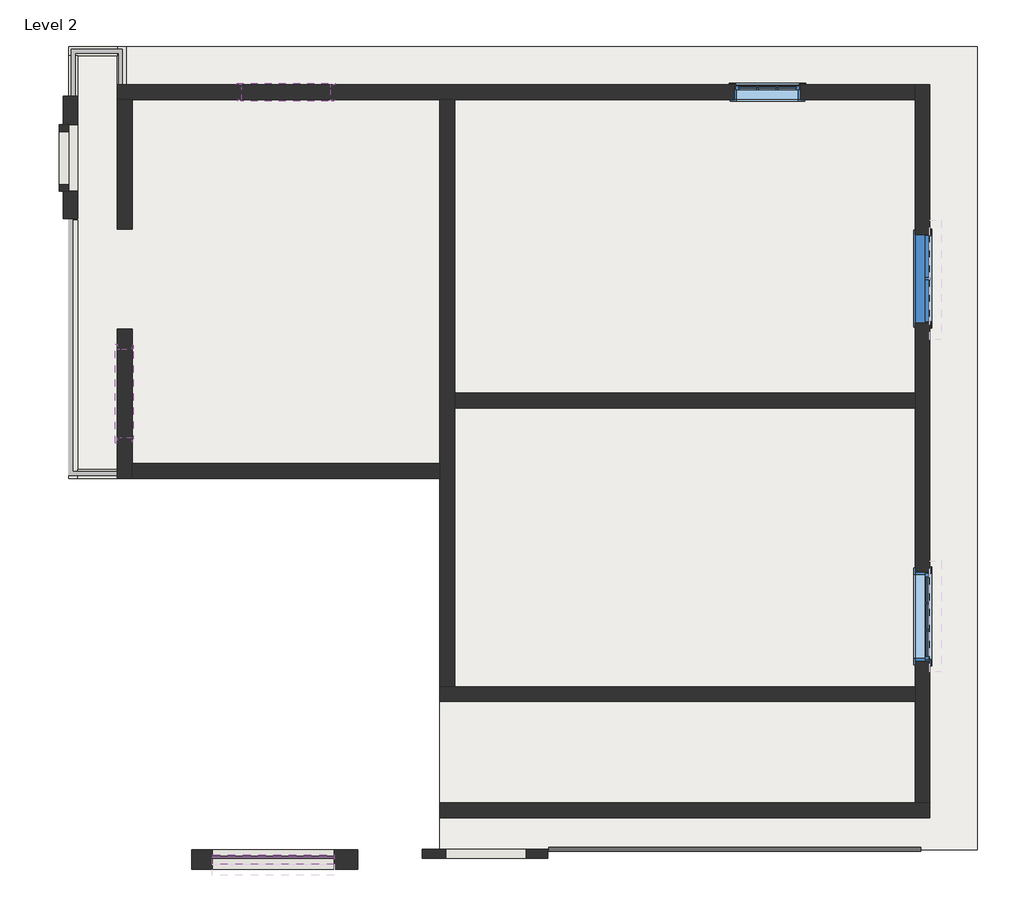
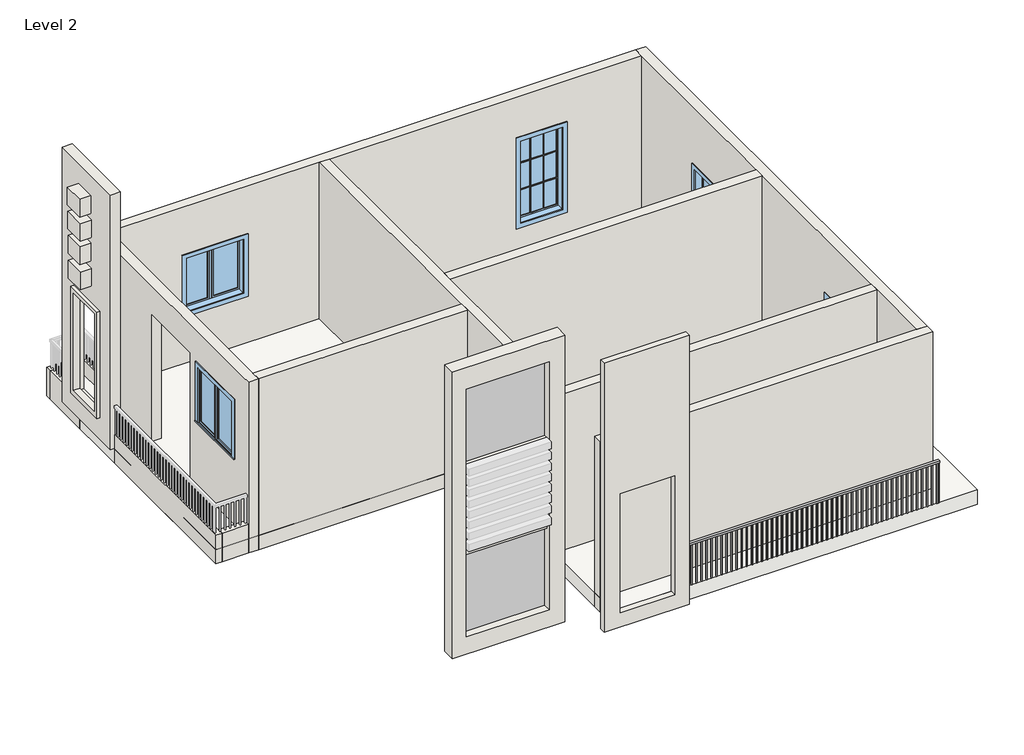
# One storey, part 1 of 2: 17 walls, 5 windows, 2 plates, 1 railing, 1 roof.
"""IFC4 building model written with IfcOpenShell, lengths in millimetres."""

from ifc_helpers import new_model, si_unit, frame, origin, place, context, project, spatial, polyline, outline, extrude, faceted_brep, transform, mapped, element, save
from components import system_panel_glazed_a1eab1ce, system_panel_glazed_1654ed80, walls_3_walls_3_431fb133, walls_4_walls_4_b785277b, window_8b323df3, window_26ecbd3e, window_0862ab64

model = new_model("IFC4")

# Units and contexts
model_context = context("Model", 3, world=origin())
ifc_project = project(units=[si_unit("LENGTHUNIT", "METRE", prefix="MILLI")], contexts=[model_context])

# Site, building, storey
site = spatial("IfcSite", under=ifc_project)
building = spatial("IfcBuilding", under=site)
storey = spatial("IfcBuildingStorey", under=building, Name="Level 2", Elevation=3657.6)

# Plates
placement = place(None, origin())
system_panel_glazed_shape = system_panel_glazed_a1eab1ce(model_context)
element("IfcPlate", 1, ObjectType="System Panel : Glazed", at=placement, inside=storey, context=model_context, shape_type="MappedRepresentation", body=[
    mapped(system_panel_glazed_shape, transform((-9639.2344883, -2764.9451776, 4624.9845939), x_axis=(1.0, 0.0, 0.0), y_axis=(0.0, 1.0, 0.0), z_axis=(0.0, 0.0, 1.0))),
])
system_panel_glazed_2_shape = system_panel_glazed_1654ed80(model_context)
element("IfcPlate", 2, ObjectType="System Panel : Glazed", at=placement, inside=storey, context=model_context, shape_type="MappedRepresentation", body=[
    mapped(system_panel_glazed_2_shape, transform((-9639.2344883, -2764.9451776, 8296.7838361), x_axis=(1.0, 0.0, 0.0), y_axis=(0.0, 1.0, 0.0), z_axis=(0.0, 0.0, 1.0))),
])

# Railing
element("IfcRailing", 3, ObjectType="Handrail - Rectangular", at=placement, inside=storey, context=model_context, shape_type="SweptSolid", body=[
    extrude(outline(polyline([(-5852.0641548, -2650.200333), (-5852.0641548, -2599.400333), (-736.6496253, -2599.400333), (-736.6496253, -2650.200333), (-5852.0641548, -2650.200333)])), frame((0.0, 0.0, 4826.0), z_axis=(0.0, 0.0, 1.0), x_axis=(1.0, 0.0, 0.0)), (0.0, 0.0, 1.0), 50.8),
    extrude(outline(polyline([(-781.5891548, -2634.325333), (-781.5891548, -2615.275333), (-762.5391548, -2615.275333), (-762.5391548, -2634.325333), (-781.5891548, -2634.325333)])), frame((0.0, 0.0, 3962.4), z_axis=(0.0, 0.0, 1.0), x_axis=(1.0, 0.0, 0.0)), (0.0, 0.0, 1.0), 863.6),
    extrude(outline(polyline([(-883.1891548, -2634.325333), (-883.1891548, -2615.275333), (-864.1391548, -2615.275333), (-864.1391548, -2634.325333), (-883.1891548, -2634.325333)])), frame((0.0, 0.0, 3962.4), z_axis=(0.0, 0.0, 1.0), x_axis=(1.0, 0.0, 0.0)), (0.0, 0.0, 1.0), 863.6),
    extrude(outline(polyline([(-984.7891548, -2634.325333), (-984.7891548, -2615.275333), (-965.7391548, -2615.275333), (-965.7391548, -2634.325333), (-984.7891548, -2634.325333)])), frame((0.0, 0.0, 3962.4), z_axis=(0.0, 0.0, 1.0), x_axis=(1.0, 0.0, 0.0)), (0.0, 0.0, 1.0), 863.6),
    extrude(outline(polyline([(-1086.3891548, -2634.325333), (-1086.3891548, -2615.275333), (-1067.3391548, -2615.275333), (-1067.3391548, -2634.325333), (-1086.3891548, -2634.325333)])), frame((0.0, 0.0, 3962.4), z_axis=(0.0, 0.0, 1.0), x_axis=(1.0, 0.0, 0.0)), (0.0, 0.0, 1.0), 863.6),
    extrude(outline(polyline([(-1187.9891548, -2634.325333), (-1187.9891548, -2615.275333), (-1168.9391548, -2615.275333), (-1168.9391548, -2634.325333), (-1187.9891548, -2634.325333)])), frame((0.0, 0.0, 3962.4), z_axis=(0.0, 0.0, 1.0), x_axis=(1.0, 0.0, 0.0)), (0.0, 0.0, 1.0), 863.6),
    extrude(outline(polyline([(-1289.5891548, -2634.325333), (-1289.5891548, -2615.275333), (-1270.5391548, -2615.275333), (-1270.5391548, -2634.325333), (-1289.5891548, -2634.325333)])), frame((0.0, 0.0, 3962.4), z_axis=(0.0, 0.0, 1.0), x_axis=(1.0, 0.0, 0.0)), (0.0, 0.0, 1.0), 863.6),
    extrude(outline(polyline([(-1391.1891548, -2634.325333), (-1391.1891548, -2615.275333), (-1372.1391548, -2615.275333), (-1372.1391548, -2634.325333), (-1391.1891548, -2634.325333)])), frame((0.0, 0.0, 3962.4), z_axis=(0.0, 0.0, 1.0), x_axis=(1.0, 0.0, 0.0)), (0.0, 0.0, 1.0), 863.6),
    extrude(outline(polyline([(-1492.7891548, -2634.325333), (-1492.7891548, -2615.275333), (-1473.7391548, -2615.275333), (-1473.7391548, -2634.325333), (-1492.7891548, -2634.325333)])), frame((0.0, 0.0, 3962.4), z_axis=(0.0, 0.0, 1.0), x_axis=(1.0, 0.0, 0.0)), (0.0, 0.0, 1.0), 863.6),
    extrude(outline(polyline([(-1594.3891548, -2634.325333), (-1594.3891548, -2615.275333), (-1575.3391548, -2615.275333), (-1575.3391548, -2634.325333), (-1594.3891548, -2634.325333)])), frame((0.0, 0.0, 3962.4), z_axis=(0.0, 0.0, 1.0), x_axis=(1.0, 0.0, 0.0)), (0.0, 0.0, 1.0), 863.6),
    extrude(outline(polyline([(-1695.9891548, -2634.325333), (-1695.9891548, -2615.275333), (-1676.9391548, -2615.275333), (-1676.9391548, -2634.325333), (-1695.9891548, -2634.325333)])), frame((0.0, 0.0, 3962.4), z_axis=(0.0, 0.0, 1.0), x_axis=(1.0, 0.0, 0.0)), (0.0, 0.0, 1.0), 863.6),
    extrude(outline(polyline([(-1797.5891548, -2634.325333), (-1797.5891548, -2615.275333), (-1778.5391548, -2615.275333), (-1778.5391548, -2634.325333), (-1797.5891548, -2634.325333)])), frame((0.0, 0.0, 3962.4), z_axis=(0.0, 0.0, 1.0), x_axis=(1.0, 0.0, 0.0)), (0.0, 0.0, 1.0), 863.6),
    extrude(outline(polyline([(-1899.1891548, -2634.325333), (-1899.1891548, -2615.275333), (-1880.1391548, -2615.275333), (-1880.1391548, -2634.325333), (-1899.1891548, -2634.325333)])), frame((0.0, 0.0, 3962.4), z_axis=(0.0, 0.0, 1.0), x_axis=(1.0, 0.0, 0.0)), (0.0, 0.0, 1.0), 863.6),
    extrude(outline(polyline([(-2000.7891548, -2634.325333), (-2000.7891548, -2615.275333), (-1981.7391548, -2615.275333), (-1981.7391548, -2634.325333), (-2000.7891548, -2634.325333)])), frame((0.0, 0.0, 3962.4), z_axis=(0.0, 0.0, 1.0), x_axis=(1.0, 0.0, 0.0)), (0.0, 0.0, 1.0), 863.6),
    extrude(outline(polyline([(-2102.3891548, -2634.325333), (-2102.3891548, -2615.275333), (-2083.3391548, -2615.275333), (-2083.3391548, -2634.325333), (-2102.3891548, -2634.325333)])), frame((0.0, 0.0, 3962.4), z_axis=(0.0, 0.0, 1.0), x_axis=(1.0, 0.0, 0.0)), (0.0, 0.0, 1.0), 863.6),
    extrude(outline(polyline([(-2203.9891548, -2634.325333), (-2203.9891548, -2615.275333), (-2184.9391548, -2615.275333), (-2184.9391548, -2634.325333), (-2203.9891548, -2634.325333)])), frame((0.0, 0.0, 3962.4), z_axis=(0.0, 0.0, 1.0), x_axis=(1.0, 0.0, 0.0)), (0.0, 0.0, 1.0), 863.6),
    extrude(outline(polyline([(-2305.5891548, -2634.325333), (-2305.5891548, -2615.275333), (-2286.5391548, -2615.275333), (-2286.5391548, -2634.325333), (-2305.5891548, -2634.325333)])), frame((0.0, 0.0, 3962.4), z_axis=(0.0, 0.0, 1.0), x_axis=(1.0, 0.0, 0.0)), (0.0, 0.0, 1.0), 863.6),
    extrude(outline(polyline([(-2407.1891548, -2634.325333), (-2407.1891548, -2615.275333), (-2388.1391548, -2615.275333), (-2388.1391548, -2634.325333), (-2407.1891548, -2634.325333)])), frame((0.0, 0.0, 3962.4), z_axis=(0.0, 0.0, 1.0), x_axis=(1.0, 0.0, 0.0)), (0.0, 0.0, 1.0), 863.6),
    extrude(outline(polyline([(-2508.7891548, -2634.325333), (-2508.7891548, -2615.275333), (-2489.7391548, -2615.275333), (-2489.7391548, -2634.325333), (-2508.7891548, -2634.325333)])), frame((0.0, 0.0, 3962.4), z_axis=(0.0, 0.0, 1.0), x_axis=(1.0, 0.0, 0.0)), (0.0, 0.0, 1.0), 863.6),
    extrude(outline(polyline([(-2610.3891548, -2634.325333), (-2610.3891548, -2615.275333), (-2591.3391548, -2615.275333), (-2591.3391548, -2634.325333), (-2610.3891548, -2634.325333)])), frame((0.0, 0.0, 3962.4), z_axis=(0.0, 0.0, 1.0), x_axis=(1.0, 0.0, 0.0)), (0.0, 0.0, 1.0), 863.6),
    extrude(outline(polyline([(-2711.9891548, -2634.325333), (-2711.9891548, -2615.275333), (-2692.9391548, -2615.275333), (-2692.9391548, -2634.325333), (-2711.9891548, -2634.325333)])), frame((0.0, 0.0, 3962.4), z_axis=(0.0, 0.0, 1.0), x_axis=(1.0, 0.0, 0.0)), (0.0, 0.0, 1.0), 863.6),
    extrude(outline(polyline([(-2813.5891548, -2634.325333), (-2813.5891548, -2615.275333), (-2794.5391548, -2615.275333), (-2794.5391548, -2634.325333), (-2813.5891548, -2634.325333)])), frame((0.0, 0.0, 3962.4), z_axis=(0.0, 0.0, 1.0), x_axis=(1.0, 0.0, 0.0)), (0.0, 0.0, 1.0), 863.6),
    extrude(outline(polyline([(-2915.1891548, -2634.325333), (-2915.1891548, -2615.275333), (-2896.1391548, -2615.275333), (-2896.1391548, -2634.325333), (-2915.1891548, -2634.325333)])), frame((0.0, 0.0, 3962.4), z_axis=(0.0, 0.0, 1.0), x_axis=(1.0, 0.0, 0.0)), (0.0, 0.0, 1.0), 863.6),
    extrude(outline(polyline([(-3016.7891548, -2634.325333), (-3016.7891548, -2615.275333), (-2997.7391548, -2615.275333), (-2997.7391548, -2634.325333), (-3016.7891548, -2634.325333)])), frame((0.0, 0.0, 3962.4), z_axis=(0.0, 0.0, 1.0), x_axis=(1.0, 0.0, 0.0)), (0.0, 0.0, 1.0), 863.6),
    extrude(outline(polyline([(-3118.3891548, -2634.325333), (-3118.3891548, -2615.275333), (-3099.3391548, -2615.275333), (-3099.3391548, -2634.325333), (-3118.3891548, -2634.325333)])), frame((0.0, 0.0, 3962.4), z_axis=(0.0, 0.0, 1.0), x_axis=(1.0, 0.0, 0.0)), (0.0, 0.0, 1.0), 863.6),
    extrude(outline(polyline([(-3219.9891548, -2634.325333), (-3219.9891548, -2615.275333), (-3200.9391548, -2615.275333), (-3200.9391548, -2634.325333), (-3219.9891548, -2634.325333)])), frame((0.0, 0.0, 3962.4), z_axis=(0.0, 0.0, 1.0), x_axis=(1.0, 0.0, 0.0)), (0.0, 0.0, 1.0), 863.6),
    extrude(outline(polyline([(-3321.5891548, -2634.325333), (-3321.5891548, -2615.275333), (-3302.5391548, -2615.275333), (-3302.5391548, -2634.325333), (-3321.5891548, -2634.325333)])), frame((0.0, 0.0, 3962.4), z_axis=(0.0, 0.0, 1.0), x_axis=(1.0, 0.0, 0.0)), (0.0, 0.0, 1.0), 863.6),
    extrude(outline(polyline([(-3423.1891548, -2634.325333), (-3423.1891548, -2615.275333), (-3404.1391548, -2615.275333), (-3404.1391548, -2634.325333), (-3423.1891548, -2634.325333)])), frame((0.0, 0.0, 3962.4), z_axis=(0.0, 0.0, 1.0), x_axis=(1.0, 0.0, 0.0)), (0.0, 0.0, 1.0), 863.6),
    extrude(outline(polyline([(-3524.7891548, -2634.325333), (-3524.7891548, -2615.275333), (-3505.7391548, -2615.275333), (-3505.7391548, -2634.325333), (-3524.7891548, -2634.325333)])), frame((0.0, 0.0, 3962.4), z_axis=(0.0, 0.0, 1.0), x_axis=(1.0, 0.0, 0.0)), (0.0, 0.0, 1.0), 863.6),
    extrude(outline(polyline([(-3626.3891548, -2634.325333), (-3626.3891548, -2615.275333), (-3607.3391548, -2615.275333), (-3607.3391548, -2634.325333), (-3626.3891548, -2634.325333)])), frame((0.0, 0.0, 3962.4), z_axis=(0.0, 0.0, 1.0), x_axis=(1.0, 0.0, 0.0)), (0.0, 0.0, 1.0), 863.6),
    extrude(outline(polyline([(-3727.9891548, -2634.325333), (-3727.9891548, -2615.275333), (-3708.9391548, -2615.275333), (-3708.9391548, -2634.325333), (-3727.9891548, -2634.325333)])), frame((0.0, 0.0, 3962.4), z_axis=(0.0, 0.0, 1.0), x_axis=(1.0, 0.0, 0.0)), (0.0, 0.0, 1.0), 863.6),
    extrude(outline(polyline([(-3829.5891548, -2634.325333), (-3829.5891548, -2615.275333), (-3810.5391548, -2615.275333), (-3810.5391548, -2634.325333), (-3829.5891548, -2634.325333)])), frame((0.0, 0.0, 3962.4), z_axis=(0.0, 0.0, 1.0), x_axis=(1.0, 0.0, 0.0)), (0.0, 0.0, 1.0), 863.6),
    extrude(outline(polyline([(-3931.1891548, -2634.325333), (-3931.1891548, -2615.275333), (-3912.1391548, -2615.275333), (-3912.1391548, -2634.325333), (-3931.1891548, -2634.325333)])), frame((0.0, 0.0, 3962.4), z_axis=(0.0, 0.0, 1.0), x_axis=(1.0, 0.0, 0.0)), (0.0, 0.0, 1.0), 863.6),
    extrude(outline(polyline([(-4032.7891548, -2634.325333), (-4032.7891548, -2615.275333), (-4013.7391548, -2615.275333), (-4013.7391548, -2634.325333), (-4032.7891548, -2634.325333)])), frame((0.0, 0.0, 3962.4), z_axis=(0.0, 0.0, 1.0), x_axis=(1.0, 0.0, 0.0)), (0.0, 0.0, 1.0), 863.6),
    extrude(outline(polyline([(-4134.3891548, -2634.325333), (-4134.3891548, -2615.275333), (-4115.3391548, -2615.275333), (-4115.3391548, -2634.325333), (-4134.3891548, -2634.325333)])), frame((0.0, 0.0, 3962.4), z_axis=(0.0, 0.0, 1.0), x_axis=(1.0, 0.0, 0.0)), (0.0, 0.0, 1.0), 863.6),
    extrude(outline(polyline([(-4235.9891548, -2634.325333), (-4235.9891548, -2615.275333), (-4216.9391548, -2615.275333), (-4216.9391548, -2634.325333), (-4235.9891548, -2634.325333)])), frame((0.0, 0.0, 3962.4), z_axis=(0.0, 0.0, 1.0), x_axis=(1.0, 0.0, 0.0)), (0.0, 0.0, 1.0), 863.6),
    extrude(outline(polyline([(-4337.5891548, -2634.325333), (-4337.5891548, -2615.275333), (-4318.5391548, -2615.275333), (-4318.5391548, -2634.325333), (-4337.5891548, -2634.325333)])), frame((0.0, 0.0, 3962.4), z_axis=(0.0, 0.0, 1.0), x_axis=(1.0, 0.0, 0.0)), (0.0, 0.0, 1.0), 863.6),
    extrude(outline(polyline([(-4439.1891548, -2634.325333), (-4439.1891548, -2615.275333), (-4420.1391548, -2615.275333), (-4420.1391548, -2634.325333), (-4439.1891548, -2634.325333)])), frame((0.0, 0.0, 3962.4), z_axis=(0.0, 0.0, 1.0), x_axis=(1.0, 0.0, 0.0)), (0.0, 0.0, 1.0), 863.6),
    extrude(outline(polyline([(-4540.7891548, -2634.325333), (-4540.7891548, -2615.275333), (-4521.7391548, -2615.275333), (-4521.7391548, -2634.325333), (-4540.7891548, -2634.325333)])), frame((0.0, 0.0, 3962.4), z_axis=(0.0, 0.0, 1.0), x_axis=(1.0, 0.0, 0.0)), (0.0, 0.0, 1.0), 863.6),
    extrude(outline(polyline([(-4642.3891548, -2634.325333), (-4642.3891548, -2615.275333), (-4623.3391548, -2615.275333), (-4623.3391548, -2634.325333), (-4642.3891548, -2634.325333)])), frame((0.0, 0.0, 3962.4), z_axis=(0.0, 0.0, 1.0), x_axis=(1.0, 0.0, 0.0)), (0.0, 0.0, 1.0), 863.6),
    extrude(outline(polyline([(-4743.9891548, -2634.325333), (-4743.9891548, -2615.275333), (-4724.9391548, -2615.275333), (-4724.9391548, -2634.325333), (-4743.9891548, -2634.325333)])), frame((0.0, 0.0, 3962.4), z_axis=(0.0, 0.0, 1.0), x_axis=(1.0, 0.0, 0.0)), (0.0, 0.0, 1.0), 863.6),
    extrude(outline(polyline([(-4845.5891548, -2634.325333), (-4845.5891548, -2615.275333), (-4826.5391548, -2615.275333), (-4826.5391548, -2634.325333), (-4845.5891548, -2634.325333)])), frame((0.0, 0.0, 3962.4), z_axis=(0.0, 0.0, 1.0), x_axis=(1.0, 0.0, 0.0)), (0.0, 0.0, 1.0), 863.6),
    extrude(outline(polyline([(-4947.1891548, -2634.325333), (-4947.1891548, -2615.275333), (-4928.1391548, -2615.275333), (-4928.1391548, -2634.325333), (-4947.1891548, -2634.325333)])), frame((0.0, 0.0, 3962.4), z_axis=(0.0, 0.0, 1.0), x_axis=(1.0, 0.0, 0.0)), (0.0, 0.0, 1.0), 863.6),
    extrude(outline(polyline([(-5048.7891548, -2634.325333), (-5048.7891548, -2615.275333), (-5029.7391548, -2615.275333), (-5029.7391548, -2634.325333), (-5048.7891548, -2634.325333)])), frame((0.0, 0.0, 3962.4), z_axis=(0.0, 0.0, 1.0), x_axis=(1.0, 0.0, 0.0)), (0.0, 0.0, 1.0), 863.6),
    extrude(outline(polyline([(-5150.3891548, -2634.325333), (-5150.3891548, -2615.275333), (-5131.3391548, -2615.275333), (-5131.3391548, -2634.325333), (-5150.3891548, -2634.325333)])), frame((0.0, 0.0, 3962.4), z_axis=(0.0, 0.0, 1.0), x_axis=(1.0, 0.0, 0.0)), (0.0, 0.0, 1.0), 863.6),
    extrude(outline(polyline([(-5251.9891548, -2634.325333), (-5251.9891548, -2615.275333), (-5232.9391548, -2615.275333), (-5232.9391548, -2634.325333), (-5251.9891548, -2634.325333)])), frame((0.0, 0.0, 3962.4), z_axis=(0.0, 0.0, 1.0), x_axis=(1.0, 0.0, 0.0)), (0.0, 0.0, 1.0), 863.6),
    extrude(outline(polyline([(-5353.5891548, -2634.325333), (-5353.5891548, -2615.275333), (-5334.5391548, -2615.275333), (-5334.5391548, -2634.325333), (-5353.5891548, -2634.325333)])), frame((0.0, 0.0, 3962.4), z_axis=(0.0, 0.0, 1.0), x_axis=(1.0, 0.0, 0.0)), (0.0, 0.0, 1.0), 863.6),
    extrude(outline(polyline([(-5455.1891548, -2634.325333), (-5455.1891548, -2615.275333), (-5436.1391548, -2615.275333), (-5436.1391548, -2634.325333), (-5455.1891548, -2634.325333)])), frame((0.0, 0.0, 3962.4), z_axis=(0.0, 0.0, 1.0), x_axis=(1.0, 0.0, 0.0)), (0.0, 0.0, 1.0), 863.6),
    extrude(outline(polyline([(-5556.7891548, -2634.325333), (-5556.7891548, -2615.275333), (-5537.7391548, -2615.275333), (-5537.7391548, -2634.325333), (-5556.7891548, -2634.325333)])), frame((0.0, 0.0, 3962.4), z_axis=(0.0, 0.0, 1.0), x_axis=(1.0, 0.0, 0.0)), (0.0, 0.0, 1.0), 863.6),
    extrude(outline(polyline([(-5658.3891548, -2634.325333), (-5658.3891548, -2615.275333), (-5639.3391548, -2615.275333), (-5639.3391548, -2634.325333), (-5658.3891548, -2634.325333)])), frame((0.0, 0.0, 3962.4), z_axis=(0.0, 0.0, 1.0), x_axis=(1.0, 0.0, 0.0)), (0.0, 0.0, 1.0), 863.6),
    extrude(outline(polyline([(-5759.9891548, -2634.325333), (-5759.9891548, -2615.275333), (-5740.9391548, -2615.275333), (-5740.9391548, -2634.325333), (-5759.9891548, -2634.325333)])), frame((0.0, 0.0, 3962.4), z_axis=(0.0, 0.0, 1.0), x_axis=(1.0, 0.0, 0.0)), (0.0, 0.0, 1.0), 863.6),
    extrude(outline(polyline([(-755.6996253, -2634.325333), (-755.6996253, -2615.275333), (-736.6496253, -2615.275333), (-736.6496253, -2634.325333), (-755.6996253, -2634.325333)])), frame((0.0, 0.0, 3962.4), z_axis=(0.0, 0.0, 1.0), x_axis=(1.0, 0.0, 0.0)), (0.0, 0.0, 1.0), 863.6),
    extrude(outline(polyline([(-5852.0641548, -2634.325333), (-5852.0641548, -2615.275333), (-5833.0141548, -2615.275333), (-5833.0141548, -2634.325333), (-5852.0641548, -2634.325333)])), frame((0.0, 0.0, 3962.4), z_axis=(0.0, 0.0, 1.0), x_axis=(1.0, 0.0, 0.0)), (0.0, 0.0, 1.0), 863.6),
])

# Roof
element("IfcRoof", 4, ObjectType="Generic - 12\"", at=placement, inside=storey, context=model_context, shape_type="SweptSolid", body=[
    extrude(outline(polyline([(-12453.9083357, 8420.5483652), (42.8916643, 8420.5483652), (42.8916643, -2628.4516348), (-7348.5083357, -2628.4516348), (-7348.5083357, 2476.9483652), (-12453.9083357, 2476.9483652), (-12453.9083357, 8420.5483652)])), frame((0.0, 0.0, 3657.6), z_axis=(0.0, 0.0, 1.0), x_axis=(1.0, 0.0, 0.0)), (0.0, 0.0, 1.0), 304.8),
])

# Walls
element("IfcWall", 5, ObjectType="Generic - 5\"", at=placement, inside=storey, context=model_context, shape_type="SweptSolid", body=[
    extrude(outline(polyline([(3657.6, -7595.2932708), (3657.6, -5868.0932708), (9420.9325813, -5868.0932708), (9420.9325813, -7595.2932708), (3657.6, -7595.2932708)]), holes=[polyline([(6512.6251814, -6163.3682708), (3962.4, -6163.3682708), (3962.4, -7272.3083357), (6512.6251814, -7272.3083357), (6512.6251814, -6163.3682708)])]), frame((0.0, -2750.326099, 0.0), z_axis=(0.0, 1.0, 0.0), x_axis=(0.0, 0.0, 1.0)), (0.0, 0.0, 1.0), 127.0),
])
element("IfcWall", 6, ObjectType="Generic - 5\"", at=placement, inside=storey, context=model_context, shape_type="Brep", body=[
    faceted_brep([(-11659.2932708, 7892.273901, 3657.6), (-11659.2932708, 8420.5483652, 3657.6), (-11659.2932708, 8420.5483652, 4267.2), (-11659.2932708, 7892.273901, 4267.2), (-11786.2932708, 7892.273901, 3657.6), (-11786.2932708, 7892.273901, 4267.2), (-11786.2932708, 8293.5483652, 4267.2), (-11786.2932708, 8420.5483652, 4267.2), (-11786.2932708, 8420.5483652, 3657.6), (-11786.2932708, 8293.5483652, 3657.6)], [[[0, 1, 2, 3]], [[4, 5, 6, 7, 8, 9]], [[1, 0, 4, 9, 8]], [[3, 2, 7, 6, 5]], [[0, 3, 5, 4]], [[2, 1, 8, 7]]]),
])
element("IfcWall", 7, ObjectType="Generic - 5\"", at=placement, inside=storey, context=model_context, shape_type="Brep", body=[
    faceted_brep([(-11786.2932708, 8420.5483652, 3657.6), (-12453.9083357, 8420.5483652, 3657.6), (-12453.9083357, 8420.5483652, 4267.2), (-11786.2932708, 8420.5483652, 4267.2), (-11786.2932708, 8293.5483652, 3657.6), (-11786.2932708, 8293.5483652, 4267.2), (-12326.9083357, 8293.5483652, 4267.2), (-12453.9083357, 8293.5483652, 4267.2), (-12453.9083357, 8293.5483652, 3657.6), (-12326.9083357, 8293.5483652, 3657.6)], [[[0, 1, 2, 3]], [[4, 5, 6, 7, 8, 9]], [[1, 0, 4, 9, 8]], [[3, 2, 7, 6, 5]], [[0, 3, 5, 4]], [[2, 1, 8, 7]]]),
])
element("IfcWall", 8, ObjectType="Generic - 5\"", at=placement, inside=storey, context=model_context, shape_type="SweptSolid", body=[
    extrude(outline(polyline([(-12453.9083357, 7251.0434239), (-12453.9083357, 8293.5483652), (-12326.9083357, 8293.5483652), (-12326.9083357, 7251.0434239), (-12453.9083357, 7251.0434239)])), frame((0.0, 0.0, 3657.6), z_axis=(0.0, 0.0, 1.0), x_axis=(1.0, 0.0, 0.0)), (0.0, 0.0, 1.0), 609.6),
])
element("IfcWall", 9, ObjectType="Generic - 5\"", at=placement, inside=storey, context=model_context, shape_type="Brep", body=[
    faceted_brep([(-12453.9083357, 6032.9483652, 3657.6), (-12453.9083357, 2476.9483652, 3657.6), (-12453.9083357, 2476.9483652, 4267.2), (-12453.9083357, 6032.9483652, 4267.2), (-12326.9083357, 6032.9483652, 3657.6), (-12326.9083357, 6032.9483652, 4267.2), (-12326.9083357, 2603.9483652, 4267.2), (-12326.9083357, 2476.9483652, 4267.2), (-12326.9083357, 2476.9483652, 3657.6), (-12326.9083357, 2603.9483652, 3657.6)], [[[0, 1, 2, 3]], [[4, 5, 6, 7, 8, 9]], [[1, 0, 4, 9, 8]], [[3, 2, 7, 6, 5]], [[0, 3, 5, 4]], [[2, 1, 8, 7]]]),
])
element("IfcWall", 10, ObjectType="Generic - 5\"", at=placement, inside=storey, context=model_context, shape_type="SweptSolid", body=[
    extrude(outline(polyline([(-11786.2932708, 2476.9483652), (-12326.9083357, 2476.9483652), (-12326.9083357, 2603.9483652), (-11786.2932708, 2603.9483652), (-11786.2932708, 2476.9483652)])), frame((0.0, 0.0, 3657.6), z_axis=(0.0, 0.0, 1.0), x_axis=(1.0, 0.0, 0.0)), (0.0, 0.0, 1.0), 609.6),
])
element("IfcWall", 11, ObjectType="Generic - 5\"", at=placement, inside=storey, context=model_context, shape_type="SweptSolid", body=[
    extrude(outline(polyline([(-8801.0344883, -2828.4451776), (-10477.4344883, -2828.4451776), (-10477.4344883, -2701.4451776), (-8801.0344883, -2701.4451776), (-8801.0344883, -2828.4451776)])), frame((0.0, 0.0, 6360.2251814), z_axis=(0.0, 0.0, 1.0), x_axis=(1.0, 0.0, 0.0)), (0.0, 0.0, 1.0), 1936.5586547),
])
element("IfcWall", 12, ObjectType="Generic - 8\"", at=placement, inside=storey, context=model_context, shape_type="Brep", body=[
    faceted_brep([(-11786.2932708, 7689.073901, 7315.2), (-11786.2932708, 7689.073901, 3657.6), (-11583.0932708, 7689.073901, 3657.6), (-7348.5083357, 7689.073901, 3657.6), (-7145.3083357, 7689.073901, 3657.6), (-813.4932708, 7689.073901, 3657.6), (-813.4932708, 7689.073901, 7315.2), (-7145.3083357, 7689.073901, 7315.2), (-7348.5083357, 7689.073901, 7315.2), (-11583.0932708, 7689.073901, 7315.2), (-2388.2932708, 7689.073901, 6386.5202928), (-2388.2932708, 7689.073901, 4557.7202928), (-3302.6932708, 7689.073901, 4557.7202928), (-3302.6932708, 7689.073901, 6386.5202928), (-8856.2008033, 7689.073901, 6244.272578), (-8856.2008033, 7689.073901, 5025.072578), (-10075.4008033, 7689.073901, 5025.072578), (-10075.4008033, 7689.073901, 6244.272578), (-11786.2932708, 7892.273901, 3657.6), (-11786.2932708, 7892.273901, 4267.2), (-11786.2932708, 7892.273901, 7315.2), (-813.4932708, 7892.273901, 7315.2), (-813.4932708, 7892.273901, 3657.6), (-11659.2932708, 7892.273901, 3657.6), (-2388.2932708, 7892.273901, 6386.5202928), (-3302.6932708, 7892.273901, 6386.5202928), (-3302.6932708, 7892.273901, 4557.7202928), (-2388.2932708, 7892.273901, 4557.7202928), (-8856.2008033, 7892.273901, 6244.272578), (-10075.4008033, 7892.273901, 6244.272578), (-10075.4008033, 7892.273901, 5025.072578), (-8856.2008033, 7892.273901, 5025.072578)], [[[0, 1, 2, 3, 4, 5, 6, 7, 8, 9], [10, 11, 12, 13], [14, 15, 16, 17]], [[18, 19, 20, 21, 22, 23], [24, 25, 26, 27], [28, 29, 30, 31]], [[5, 4, 3, 2, 1, 18, 23, 22]], [[0, 9, 8, 7, 6, 21, 20]], [[6, 5, 22, 21]], [[0, 20, 19, 18, 1]], [[11, 10, 24, 27]], [[12, 11, 27, 26]], [[13, 12, 26, 25]], [[10, 13, 25, 24]], [[15, 14, 28, 31]], [[16, 15, 31, 30]], [[17, 16, 30, 29]], [[14, 17, 29, 28]]]),
])
element("IfcWall", 13, ObjectType="Generic - 8\"", at=placement, inside=storey, context=model_context, shape_type="Brep", body=[
    faceted_brep([(-11583.0932708, 2476.9483652, 7315.2), (-11583.0932708, 2476.9483652, 3657.6), (-11583.0932708, 2578.5483652, 3657.6), (-11583.0932708, 2680.1483652, 3657.6), (-11583.0932708, 4533.8772304, 3657.6), (-11583.0932708, 4533.8772304, 6705.6), (-11583.0932708, 5905.4772304, 6705.6), (-11583.0932708, 5905.4772304, 3657.6), (-11583.0932708, 7689.073901, 3657.6), (-11583.0932708, 7689.073901, 7315.2), (-11583.0932708, 2680.1483652, 7315.2), (-11583.0932708, 4254.9483652, 6584.0797977), (-11583.0932708, 4254.9483652, 5364.8797977), (-11583.0932708, 3035.7483652, 5364.8797977), (-11583.0932708, 3035.7483652, 6584.0797977), (-11786.2932708, 2476.9483652, 3657.6), (-11786.2932708, 2476.9483652, 4267.2), (-11786.2932708, 2476.9483652, 7315.2), (-11786.2932708, 2680.1483652, 7315.2), (-11786.2932708, 7689.073901, 7315.2), (-11786.2932708, 7689.073901, 3657.6), (-11786.2932708, 5905.4772304, 3657.6), (-11786.2932708, 5905.4772304, 6705.6), (-11786.2932708, 4533.8772304, 6705.6), (-11786.2932708, 4533.8772304, 3657.6), (-11786.2932708, 2603.9483652, 3657.6), (-11786.2932708, 2578.5483652, 3657.6), (-11786.2932708, 4254.9483652, 6584.0797977), (-11786.2932708, 3035.7483652, 6584.0797977), (-11786.2932708, 3035.7483652, 5364.8797977), (-11786.2932708, 4254.9483652, 5364.8797977)], [[[0, 1, 2, 3, 4, 5, 6, 7, 8, 9, 10], [11, 12, 13, 14]], [[15, 16, 17, 18, 19, 20, 21, 22, 23, 24, 25, 26], [27, 28, 29, 30]], [[0, 17, 16, 15, 1]], [[8, 20, 19, 9]], [[12, 11, 27, 30]], [[13, 12, 30, 29]], [[14, 13, 29, 28]], [[11, 14, 28, 27]], [[0, 10, 9, 19, 18, 17]], [[4, 3, 2, 1, 15, 26, 25, 24]], [[5, 4, 24, 23]], [[6, 5, 23, 22]], [[7, 6, 22, 21]], [[8, 7, 21, 20]]]),
])
element("IfcWall", 14, ObjectType="Generic - 8\"", at=placement, inside=storey, context=model_context, shape_type="Brep", body=[
    faceted_brep([(-610.2932708, -1988.326099, 3657.6), (-813.4932708, -1988.326099, 3657.6), (-7348.5083357, -1988.326099, 3657.6), (-7348.5083357, -1988.326099, 7315.2), (-813.4932708, -1988.326099, 7315.2), (-610.2932708, -1988.326099, 7315.2), (-610.2932708, -2191.526099, 3657.6), (-610.2932708, -2191.526099, 7315.2), (-7348.5083357, -2191.526099, 7315.2), (-7348.5083357, -2191.526099, 3657.6)], [[[0, 1, 2, 3, 4, 5]], [[6, 7, 8, 9]], [[2, 1, 0, 6, 9]], [[3, 2, 9, 8]], [[5, 4, 3, 8, 7]], [[0, 5, 7, 6]]]),
])
element("IfcWall", 15, ObjectType="Generic - 8\"", at=placement, inside=storey, context=model_context, shape_type="Brep", body=[
    faceted_brep([(-813.4932708, 7892.273901, 3657.6), (-813.4932708, 7689.073901, 3657.6), (-813.4932708, 3650.473901, 3657.6), (-813.4932708, 3447.273901, 3657.6), (-813.4932708, -388.126099, 3657.6), (-813.4932708, -591.326099, 3657.6), (-813.4932708, -1988.326099, 3657.6), (-813.4932708, -1988.326099, 7315.2), (-813.4932708, -591.326099, 7315.2), (-813.4932708, -388.126099, 7315.2), (-813.4932708, 3447.273901, 7315.2), (-813.4932708, 3650.473901, 7315.2), (-813.4932708, 7689.073901, 7315.2), (-813.4932708, 7892.273901, 7315.2), (-813.4932708, -32.526099, 6096.0), (-813.4932708, -32.526099, 4572.0), (-813.4932708, 1186.673901, 4572.0), (-813.4932708, 1186.673901, 6096.0), (-813.4932708, 4615.673901, 6045.2), (-813.4932708, 4615.673901, 4826.0), (-813.4932708, 5834.873901, 4826.0), (-813.4932708, 5834.873901, 6045.2), (-610.2932708, 7892.273901, 3657.6), (-610.2932708, 7892.273901, 7315.2), (-610.2932708, -1988.326099, 7315.2), (-610.2932708, -1988.326099, 3657.6), (-610.2932708, -32.526099, 6096.0), (-610.2932708, 1186.673901, 6096.0), (-610.2932708, 1186.673901, 4572.0), (-610.2932708, -32.526099, 4572.0), (-610.2932708, 4615.673901, 6045.2), (-610.2932708, 5834.873901, 6045.2), (-610.2932708, 5834.873901, 4826.0), (-610.2932708, 4615.673901, 4826.0)], [[[0, 1, 2, 3, 4, 5, 6, 7, 8, 9, 10, 11, 12, 13], [14, 15, 16, 17], [18, 19, 20, 21]], [[22, 23, 24, 25], [26, 27, 28, 29], [30, 31, 32, 33]], [[6, 5, 4, 3, 2, 1, 0, 22, 25]], [[13, 12, 11, 10, 9, 8, 7, 24, 23]], [[0, 13, 23, 22]], [[7, 6, 25, 24]], [[15, 14, 26, 29]], [[16, 15, 29, 28]], [[17, 16, 28, 27]], [[14, 17, 27, 26]], [[19, 18, 30, 33]], [[20, 19, 33, 32]], [[21, 20, 32, 31]], [[18, 21, 31, 30]]]),
])
element("IfcWall", 16, ObjectType="Generic - 8\"", at=placement, inside=storey, context=model_context, shape_type="Brep", body=[
    faceted_brep([(-813.4932708, -388.126099, 3657.6), (-7145.3083357, -388.126099, 3657.6), (-7348.5083357, -388.126099, 3657.6), (-7348.5083357, -388.126099, 7315.2), (-7145.3083357, -388.126099, 7315.2), (-813.4932708, -388.126099, 7315.2), (-813.4932708, -591.326099, 3657.6), (-813.4932708, -591.326099, 7315.2), (-7348.5083357, -591.326099, 7315.2), (-7348.5083357, -591.326099, 3657.6)], [[[0, 1, 2, 3, 4, 5]], [[6, 7, 8, 9]], [[2, 1, 0, 6, 9]], [[5, 4, 3, 8, 7]], [[0, 5, 7, 6]], [[3, 2, 9, 8]]]),
])
element("IfcWall", 17, ObjectType="Generic - 8\"", at=placement, inside=storey, context=model_context, shape_type="Brep", body=[
    faceted_brep([(-7145.3083357, -388.126099, 3657.6), (-7145.3083357, 3447.273901, 3657.6), (-7145.3083357, 3650.473901, 3657.6), (-7145.3083357, 7689.073901, 3657.6), (-7145.3083357, 7689.073901, 7315.2), (-7145.3083357, 3650.473901, 7315.2), (-7145.3083357, 3447.273901, 7315.2), (-7145.3083357, -388.126099, 7315.2), (-7348.5083357, -388.126099, 3657.6), (-7348.5083357, -388.126099, 7315.2), (-7348.5083357, 2476.9483652, 7315.2), (-7348.5083357, 2680.1483652, 7315.2), (-7348.5083357, 7689.073901, 7315.2), (-7348.5083357, 7689.073901, 3657.6), (-7348.5083357, 2680.1483652, 3657.6), (-7348.5083357, 2476.9483652, 3657.6)], [[[0, 1, 2, 3, 4, 5, 6, 7]], [[8, 9, 10, 11, 12, 13, 14, 15]], [[3, 2, 1, 0, 8, 15, 14, 13]], [[7, 6, 5, 4, 12, 11, 10, 9]], [[0, 7, 9, 8]], [[4, 3, 13, 12]]]),
])
element("IfcWall", 18, ObjectType="Generic - 8\"", at=placement, inside=storey, context=model_context, shape_type="Brep", body=[
    faceted_brep([(-7348.5083357, 2680.1483652, 3657.6), (-11583.0932708, 2680.1483652, 3657.6), (-11583.0932708, 2680.1483652, 7315.2), (-7366.6932708, 2680.1483652, 7315.2), (-7348.5083357, 2680.1483652, 7315.2), (-7348.5083357, 2476.9483652, 3657.6), (-7348.5083357, 2476.9483652, 7315.2), (-7366.6932708, 2476.9483652, 7315.2), (-11583.0932708, 2476.9483652, 7315.2), (-11583.0932708, 2476.9483652, 3657.6)], [[[0, 1, 2, 3, 4]], [[5, 6, 7, 8, 9]], [[1, 0, 5, 9]], [[4, 3, 2, 8, 7, 6]], [[0, 4, 6, 5]], [[1, 9, 8, 2]]]),
])
element("IfcWall", 19, ObjectType="Generic - 8\"", at=placement, inside=storey, context=model_context, shape_type="SweptSolid", body=[
    extrude(outline(polyline([(-813.4932708, 3447.273901), (-7145.3083357, 3447.273901), (-7145.3083357, 3650.473901), (-813.4932708, 3650.473901), (-813.4932708, 3447.273901)])), frame((0.0, 0.0, 3657.6), z_axis=(0.0, 0.0, 1.0), x_axis=(1.0, 0.0, 0.0)), (0.0, 0.0, 1.0), 3657.6),
])
walls_3_walls_3_shape = walls_3_walls_3_431fb133(model_context)
element("IfcWall", 20, ObjectType="Walls 3 : Walls 3", at=placement, inside=storey, context=model_context, shape_type="MappedRepresentation", body=[
    mapped(walls_3_walls_3_shape, transform((0.0, 0.0, 0.0), x_axis=(1.0, 0.0, 0.0), y_axis=(0.0, 1.0, 0.0), z_axis=(0.0, 0.0, 1.0))),
])
walls_4_walls_4_shape = walls_4_walls_4_b785277b(model_context)
element("IfcWall", 21, ObjectType="Walls 4 : Walls 4", at=placement, inside=storey, context=model_context, shape_type="MappedRepresentation", body=[
    mapped(walls_4_walls_4_shape, transform((0.0, 0.0, 0.0), x_axis=(1.0, 0.0, 0.0), y_axis=(0.0, 1.0, 0.0), z_axis=(0.0, 0.0, 1.0))),
])

# Windows
window_shape = window_8b323df3(model_context)
element("IfcWindow", 22, ObjectType="Casement 3x3 with Trim : 36\" x 72\"", at=placement, inside=storey, context=model_context, shape_type="MappedRepresentation", body=[
    mapped(window_shape, transform((-2845.4932708, 7790.673901, 4252.9202928), x_axis=(1.0, 0.0, 0.0), y_axis=(0.0, 1.0, 0.0), z_axis=(0.0, 0.0, 1.0))),
])
window_2_shape = window_26ecbd3e(model_context)
element("IfcWindow", 23, ObjectType="Casement 3x3 with Trim : 48\" x 60\"", at=placement, inside=storey, context=model_context, shape_type="MappedRepresentation", body=[
    mapped(window_2_shape, transform((-711.8932708, 577.073901, 3657.6), x_axis=(0.0, -1.0, 0.0), y_axis=(1.0, 0.0, 0.0), z_axis=(0.0, 0.0, 1.0))),
])
window_3_shape = window_0862ab64(model_context)
element("IfcWindow", 24, ObjectType="Casement Dbl with Trim.0001 : 48\" x 48\"", at=placement, inside=storey, context=model_context, shape_type="MappedRepresentation", body=[
    mapped(window_3_shape, transform((-11665.6432708, 3645.3483652, 4450.4797977), x_axis=(0.0, 1.0, 0.0), y_axis=(-1.0, 0.0, 0.0), z_axis=(0.0, 0.0, 1.0))),
])
element("IfcWindow", 25, ObjectType="Casement Dbl with Trim.0001 : 48\" x 48\"", at=placement, inside=storey, context=model_context, shape_type="MappedRepresentation", body=[
    mapped(window_3_shape, transform((-730.9432708, 5225.273901, 3911.6), x_axis=(0.0, -1.0, 0.0), y_axis=(1.0, 0.0, 0.0), z_axis=(0.0, 0.0, 1.0))),
])
element("IfcWindow", 26, ObjectType="Casement Dbl with Trim.0001 : 48\" x 48\"", at=placement, inside=storey, context=model_context, shape_type="MappedRepresentation", body=[
    mapped(window_3_shape, transform((-9465.8008033, 7771.623901, 4110.672578), x_axis=(1.0, 0.0, 0.0), y_axis=(0.0, 1.0, 0.0), z_axis=(0.0, 0.0, 1.0))),
])

save(model, "model.ifc")

# Revit data of these elements
# Type "System Panel : Glazed"
#   Construction Type Id = "GSP4R"
#   Analytic Construction = "1/8 in Pilkington single glazing"
#   Visual Light Transmittance = 0.9
#   Solar Heat Gain Coefficient = 0.86
#   Heat Transfer Coefficient (U) = 1.18115 BTU/(h·ft²·°F)
# Type "Handrail - Rectangular"
#   Assembly Code = "C2010400"
#   built-in parameter 1008612 = 0.0416667 (stored number, unit not read)
#   built-in parameter 1008611 = 0.0416667 (stored number, unit not read)
#   built-in parameter 1008609 = 0.333333 (stored number, unit not read)
#   built-in parameter 1008604 = 0.166667 (stored number, unit not read)
#   built-in parameter 1008603 = 0.166667 (stored number, unit not read)
#   Railing Height = 3' - 0"
#   built-in parameter 1008630 = 2
#   built-in parameter 1008610 = 2
#   built-in parameter 1008618 = Baluster - Square : 3/4"
# Type "Generic - 12\""
#   Assembly Code = "B1020"
#   Layers, outside or top first: 1' - 0" no material (function 1)
# Type "Generic - 5\""
#   Assembly Code = "B2010"
#   Layers, outside or top first: 0' - 5" no material (function 1)
# Type "Generic - 8\""
#   Assembly Code = "B2010"
#   Layers, outside or top first: 0' - 8" no material (function 1)
# Type "Casement 3x3 with Trim : 36\" x 72\""
#   Type Mark = "15"
#   Construction Type Id = "GSP4R"
#   Assembly Code = "B2020100"
#   Analytic Construction = "1/8 in Pilkington single glazing"
#   Visual Light Transmittance = 0.9
#   Solar Heat Gain Coefficient = 0.78
#   Heat Transfer Coefficient (U) = 0.6496 BTU/(h·ft²·°F)
#   Height = 6' - 0"
#   Default Sill Height = 1' - 0"
#   Trim Projection - Ext. = 0' - 0 1/2"
#   Trim Projection - Int. = 0' - 0 3/4"
#   Trim Width - Exterior = 0' - 3 1/2"
#   Trim Width - Interior = 0' - 3 1/2"
#   Width = 3' - 0"
#   Window Inset = 0' - 0 3/4"
#   Define Thermal Properties by = 1
#   Glass Pane Material = Glass
#   Sash Material = Sash
#   Trim Exterior Material = Trim
#   Trim Interior Material = Trim
#   Wall Closure = (empty or 0)
# Type "Casement 3x3 with Trim : 48\" x 60\""
#   Type Mark = "13"
#   Construction Type Id = "GSP4R"
#   Assembly Code = "B2020100"
#   Analytic Construction = "1/8 in Pilkington single glazing"
#   Visual Light Transmittance = 0.9
#   Solar Heat Gain Coefficient = 0.78
#   Heat Transfer Coefficient (U) = 0.6496 BTU/(h·ft²·°F)
#   Height = 5' - 0"
#   Default Sill Height = 3' - 0"
#   Trim Projection - Ext. = 0' - 0 1/2"
#   Trim Projection - Int. = 0' - 0 3/4"
#   Trim Width - Exterior = 0' - 3 1/2"
#   Trim Width - Interior = 0' - 3 1/2"
#   Width = 4' - 0"
#   Window Inset = 0' - 0 3/4"
#   Define Thermal Properties by = 1
#   Glass Pane Material = Glass
#   Sash Material = Sash
#   Trim Exterior Material = Trim
#   Trim Interior Material = Trim
#   Wall Closure = (empty or 0)
# Type "Casement Dbl with Trim.0001 : 48\" x 48\""
#   Type Mark = "10"
#   Construction Type Id = "GSP4R"
#   Assembly Code = "B2020100"
#   Analytic Construction = "1/8 in Pilkington single glazing"
#   Visual Light Transmittance = 0.9
#   Solar Heat Gain Coefficient = 0.78
#   Heat Transfer Coefficient (U) = 0.6496 BTU/(h·ft²·°F)
#   Height = 4' - 0"
#   Default Sill Height = 3' - 0"
#   Trim Projection - Ext. = 0' - 0 1/2"
#   Trim Projection - Int. = 0' - 0 3/4"
#   Trim Width - Exterior = 0' - 3 1/2"
#   Trim Width - Interior = 0' - 3 1/2"
#   Width = 4' - 0"
#   Window Inset = 0' - 0 3/4"
#   Define Thermal Properties by = 1
#   Glass Pane Material = Glass
#   Sash Material = Sash
#   Trim Exterior Material = Trim
#   Trim Interior Material = Trim
#   Wall Closure = (empty or 0)
# Elements 1, 2 (IfcPlate, "System Panel : Glazed")
#   Phase Created = New Construction
#   Materials on its faces: "Glass"
# Element 3 (IfcRailing, "Handrail - Rectangular")
#   built-in parameter 1008621 = 1 (stored number, unit not read)
#   Phase Created = New Construction
# Element 4 (IfcRoof, "Generic - 12\"")
#   built-in parameter 1001705 = 13 (stored number, unit not read)
#   built-in parameter 1001710 = 33615
#   Phase Created = New Construction
#   Materials on its faces: "Default Roof"
# Element 5 (IfcWall, "Generic - 5\"")
#   Top Offset = 6' - 10.90286"
#   Base Offset = 0' - 0"
#   wall height = 18' - 10.90286"
#   Phase Created = New Construction
#   Base Constraint = Level 2
#   Top Constraint = Level 3
#   Materials on its faces: "Default Wall"
# Elements 6, 7, 8, 9, 10 (IfcWall, "Generic - 5\"")
#   Top Offset = -10' - 0"
#   Base Offset = 0' - 0"
#   wall height = 2' - 0"
#   Phase Created = New Construction
#   Base Constraint = Level 2
#   Top Constraint = Level 3
#   Materials on its faces: "Default Wall"
# Element 11 (IfcWall, "Generic - 5\"")
#   built-in parameter 1001111 = 8' - 10.40257"
#   Top Offset = 3' - 2.64503"
#   Base Offset = 8' - 10.40257"
#   wall height = 6' - 4.24247"
#   Phase Created = New Construction
#   Base Constraint = Level 2
#   Top Constraint = Level 3
#   Materials on its faces: "Default Wall"
# Elements 12, 13, 14, 15, 16, 17, 18, 19 (IfcWall, "Generic - 8\"")
#   Top Offset = 0' - 0"
#   Base Offset = 0' - 0"
#   Unconnected Height = 12' - 0"
#   wall height = 12' - 0"
#   Phase Created = New Construction
#   Base Constraint = Level 2
#   Materials on its faces: "Default Wall"
# Element 20 (IfcWall, "Walls 3 : Walls 3")
#   Phase Created = New Construction
#   Materials on its faces: "Default Wall"
# Element 21 (IfcWall, "Walls 4 : Walls 4")
#   Phase Created = New Construction
#   Materials on its faces: "Default Wall"
# Element 22 (IfcWindow, "Casement 3x3 with Trim : 36\" x 72\"")
#   Mark = "8"
#   Phase Created = New Construction
#   Materials on its faces: "Sash", "Glass", "Trim"
# Element 23 (IfcWindow, "Casement 3x3 with Trim : 48\" x 60\"")
#   Mark = "4"
#   Phase Created = New Construction
#   Materials on its faces: "Sash", "Glass", "Trim"
# Element 24 (IfcWindow, "Casement Dbl with Trim.0001 : 48\" x 48\"")
#   Mark = "2"
#   Phase Created = New Construction
#   Materials on its faces: "Sash", "Trim", "Glass"
# Element 25 (IfcWindow, "Casement Dbl with Trim.0001 : 48\" x 48\"")
#   Mark = "7"
#   Phase Created = New Construction
#   Materials on its faces: "Sash", "Trim", "Glass"
# Element 26 (IfcWindow, "Casement Dbl with Trim.0001 : 48\" x 48\"")
#   Mark = "11"
#   Phase Created = New Construction
#   Materials on its faces: "Sash", "Trim", "Glass"
# Materials
#   "Glass": class "Glass", colour RGB 0 128 192, transparency 0.75, Description = "Soda Lime Glass", Cost = 0
#   "Sash": class "Wood", colour RGB 224 178 126, transparency 0
#   "Trim": class "Wood", colour RGB 224 178 126, transparency 0
#   "Default Roof": colour RGB 88 101 114, transparency 0
#   "Default Wall": colour RGB 128 128 128, transparency 0
